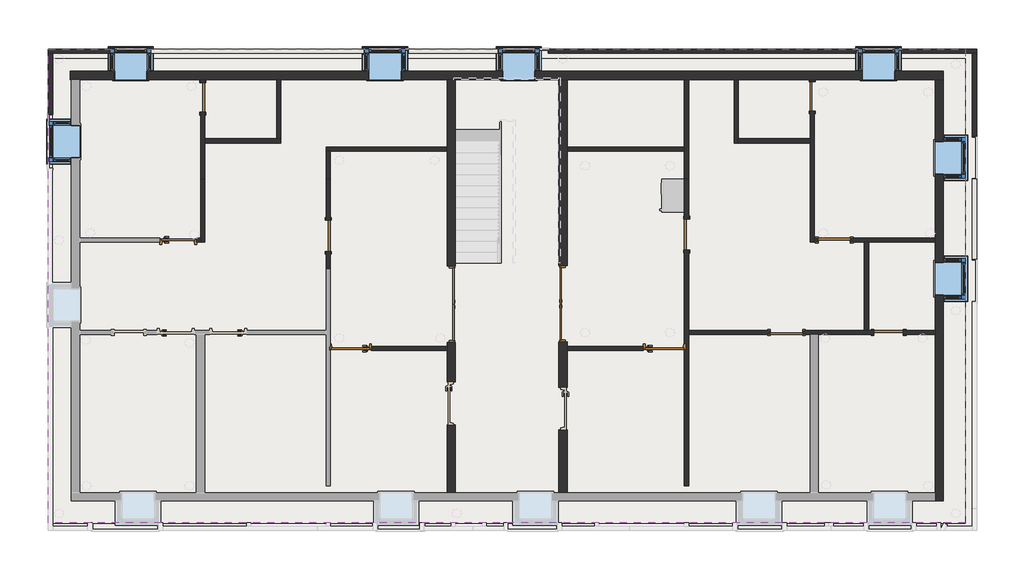
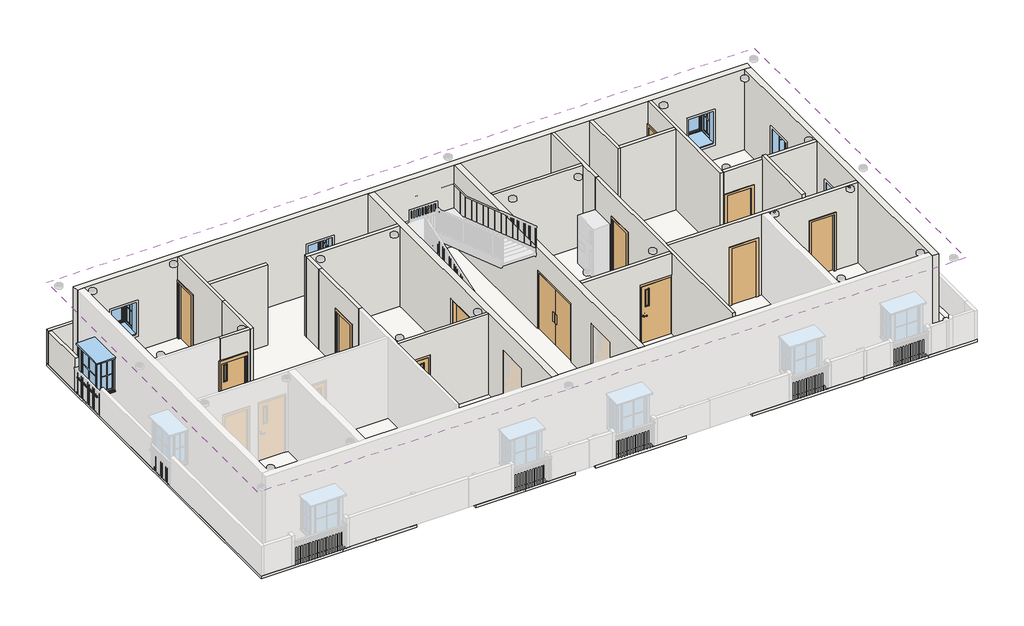
# One storey, part 2 of 7: 32 walls, 12 doors, 7 windows, 2 slabs, 1 covering.
"""IFC4 building model written with IfcOpenShell, lengths in millimetres."""

from ifc_helpers import new_model, si_unit, frame, origin, place, context, project, spatial, polyline, outline, extrude, faceted_brep, transform, mapped, element, save
from components import door_2c854dd0, door_cf1f2706, door_4f5842df, door_passage_single_vision_lite_3_x7_440dd290, door_70e57c00, door_700d3439, door_8cb1b8a7, door_38851409, door_d141acb4, window_bay_casement_box_90_degree_angle_center_fixed_4_x3_2dea7aab

model = new_model("IFC4")

# Units and contexts
model_context = context("Model", 3, world=origin())
ifc_project = project(units=[si_unit("LENGTHUNIT", "METRE", prefix="MILLI")], contexts=[model_context])

# Site, building, storey
site = spatial("IfcSite", under=ifc_project)
building = spatial("IfcBuilding", under=site)
storey = spatial("IfcBuildingStorey", under=building, Elevation=3200.4)

# Covering
placement = place(None, origin())
element("IfcCovering", 1, ObjectType="2' x 4' ACT System", at=placement, inside=storey, context=model_context, shape_type="SweptSolid", body=[
    extrude(outline(polyline([(12235.5012075, 8470.0067329), (12235.5012075, -4623.6932193), (-13088.8067989, -4623.6932193), (-13088.8067989, 8470.0067329), (12235.5012075, 8470.0067329)])), frame((0.0, 0.0, 6248.4), z_axis=(0.0, 0.0, 1.0), x_axis=(1.0, 0.0, 0.0)), (0.0, 0.0, 1.0), 57.15),
])

# Doors
door_shape = door_2c854dd0(model_context)
element("IfcDoor", 2, ObjectType="Door-Passage-Double-Flush-Dbl_Acting : 6'79\" X 84\"", at=placement, inside=storey, context=model_context, shape_type="MappedRepresentation", body=[
    mapped(door_shape, transform((-1969.4487998, 1424.4578621, 3200.4), x_axis=(0.0, -1.0, 0.0), y_axis=(1.0, 0.0, 0.0), z_axis=(0.0, 0.0, 1.0))),
])
element("IfcDoor", 3, ObjectType="Door-Passage-Double-Flush-Dbl_Acting : 6'79\" X 84\"", at=placement, inside=storey, context=model_context, shape_type="MappedRepresentation", body=[
    mapped(door_shape, transform((1128.8432011, 1434.2067807, 3200.4), x_axis=(0.0, 1.0, 0.0), y_axis=(-1.0, 0.0, 0.0), z_axis=(0.0, 0.0, 1.0))),
])
door_2_shape = door_cf1f2706(model_context)
element("IfcDoor", 4, ObjectType="Door-Passage-Single-Vision_Lite : 3'6\"X7' 2", at=placement, inside=storey, context=model_context, shape_type="MappedRepresentation", body=[
    mapped(door_2_shape, transform((-4750.7487995, 211.6078621, 3200.4), x_axis=(-1.0, 0.0, 0.0), y_axis=(0.0, -1.0, 0.0), z_axis=(0.0, 0.0, 1.0))),
])
door_3_shape = door_4f5842df(model_context)
element("IfcDoor", 5, ObjectType="Door-Passage-Single-Vision_Lite : 3'6\"X7' 2", at=placement, inside=storey, context=model_context, shape_type="MappedRepresentation", body=[
    mapped(door_3_shape, transform((3923.3512082, 211.6078621, 3200.4), x_axis=(1.0, 0.0, 0.0), y_axis=(0.0, 1.0, 0.0), z_axis=(0.0, 0.0, 1.0))),
])
door_passage_single_vision_lite_3_x7_shape = door_passage_single_vision_lite_3_x7_440dd290(model_context)
element("IfcDoor", 6, ObjectType="Door-Passage-Single-Vision_Lite : 3'X7'", at=placement, inside=storey, context=model_context, shape_type="MappedRepresentation", body=[
    mapped(door_passage_single_vision_lite_3_x7_shape, transform((-9501.8462614, 3186.8067332, 3200.4), x_axis=(1.0, 0.0, 0.0), y_axis=(0.0, 1.0, 0.0), z_axis=(0.0, 0.0, 1.0))),
])
door_4_shape = door_70e57c00(model_context)
element("IfcDoor", 7, ObjectType="Single-Flush : 2'10\" x 7'", at=placement, inside=storey, context=model_context, shape_type="MappedRepresentation", body=[
    mapped(door_4_shape, transform((-5360.3487995, 3313.8067802, 3200.4), x_axis=(0.0, -1.0, 0.0), y_axis=(1.0, 0.0, 0.0), z_axis=(0.0, 0.0, 1.0))),
])
door_5_shape = door_700d3439(model_context)
element("IfcDoor", 8, ObjectType="Single-Flush : 2'10\" x 7'", at=placement, inside=storey, context=model_context, shape_type="MappedRepresentation", body=[
    mapped(door_5_shape, transform((4532.9512082, 3351.906733, 3200.4), x_axis=(0.0, -1.0, 0.0), y_axis=(1.0, 0.0, 0.0), z_axis=(0.0, 0.0, 1.0))),
])
door_6_shape = door_8cb1b8a7(model_context)
element("IfcDoor", 9, ObjectType="Single-Flush : 2'11\"x 7'", at=placement, inside=storey, context=model_context, shape_type="MappedRepresentation", body=[
    mapped(door_6_shape, transform((8609.6512079, 3193.1567332, 3200.4), x_axis=(-1.0, 0.0, 0.0), y_axis=(0.0, -1.0, 0.0), z_axis=(0.0, 0.0, 1.0))),
])
element("IfcDoor", 10, ObjectType="Single-Flush : 2'11\"x 7'", at=placement, inside=storey, context=model_context, shape_type="MappedRepresentation", body=[
    mapped(door_6_shape, transform((7295.2012079, 640.4567334, 3200.4), x_axis=(1.0, 0.0, 0.0), y_axis=(0.0, 1.0, 0.0), z_axis=(0.0, 0.0, 1.0))),
])
door_7_shape = door_38851409(model_context)
element("IfcDoor", 11, ObjectType="Single-Flush : 2'8\"x 7'", at=placement, inside=storey, context=model_context, shape_type="MappedRepresentation", body=[
    mapped(door_7_shape, transform((-8827.4487992, 7136.5067329, 3200.4), x_axis=(0.0, 1.0, 0.0), y_axis=(-1.0, 0.0, 0.0), z_axis=(0.0, 0.0, 1.0))),
])
element("IfcDoor", 12, ObjectType="Single-Flush : 2'8\"x 7'", at=placement, inside=storey, context=model_context, shape_type="MappedRepresentation", body=[
    mapped(door_7_shape, transform((10111.5098918, 640.4567334, 3200.4), x_axis=(-1.0, 0.0, 0.0), y_axis=(0.0, -1.0, 0.0), z_axis=(0.0, 0.0, 1.0))),
])
door_8_shape = door_d141acb4(model_context)
element("IfcDoor", 13, ObjectType="Single-Flush : 2'8\"x 7'", at=placement, inside=storey, context=model_context, shape_type="MappedRepresentation", body=[
    mapped(door_8_shape, transform((8000.0512079, 7167.840939, 3200.4), x_axis=(0.0, 1.0, 0.0), y_axis=(-1.0, 0.0, 0.0), z_axis=(0.0, 0.0, 1.0))),
])

# Slabs
element("IfcSlab", 14, ObjectType="LW Concrete on Metal Deck", at=placement, inside=storey, context=model_context, shape_type="SweptSolid", body=[
    extrude(outline(polyline([(12235.5012075, 8203.3067329), (12235.5012075, -4623.6932193), (-12973.9987925, -4623.6932193), (-12973.9987925, 8203.3067329), (12235.5012075, 8203.3067329)])), frame((0.0, 0.0, 3095.625), z_axis=(0.0, 0.0, 1.0), x_axis=(1.0, 0.0, 0.0)), (0.0, 0.0, 1.0), 104.775),
])
element("IfcSlab", 15, ObjectType="LW Concrete on Metal Deck", at=placement, inside=storey, context=model_context, shape_type="SweptSolid", body=[
    extrude(outline(polyline([(12540.3012043, 8470.0067329), (12540.3012043, -4826.8932661), (10789.5617205, -4826.8932661), (8463.6012082, -4826.8932661), (8463.6012082, -3785.4932193), (8457.2512082, -3785.4932193), (8457.2512082, -4826.8932661), (4475.8012082, -4826.8932661), (4475.8012082, -3785.4932193), (2113.6012002, -3785.4932193), (2113.6012002, -4826.8932661), (-1112.1987998, -4826.8932661), (-1112.1987998, -3785.4932193), (-1848.7987998, -3785.4932193), (-1848.7987998, -4826.8932661), (-3627.0527957, -4826.8932661), (-5417.4987995, -4826.8932661), (-5417.4987995, -3785.4932193), (-7513.2527957, -3785.4932193), (-7513.2527957, -4826.8932661), (-8961.0527957, -4826.8932661), (-10167.8067989, -4826.8932661), (-13088.8067989, -4826.8932661), (-13088.8067989, 8470.0067329), (12540.3012043, 8470.0067329)])), frame((0.0, 0.0, 3095.625), z_axis=(0.0, 0.0, 1.0), x_axis=(1.0, 0.0, 0.0)), (0.0, 0.0, 1.0), 104.775),
])

# Walls
element("IfcWall", 16, ObjectType="Generic - 4.5\"", at=placement, inside=storey, context=model_context, shape_type="Brep", body=[
    faceted_brep([(-8884.5987992, 4875.906733, 3200.4), (-8884.5987992, 3250.3067332, 3200.4), (-8884.5987992, 3136.0067332, 3200.4), (-8884.5987992, 3136.0067332, 6248.4), (-8884.5987992, 3250.3067332, 6248.4), (-8884.5987992, 4875.906733, 6248.4), (-8770.2987992, 4875.906733, 3200.4), (-8770.2987992, 4875.906733, 6248.4), (-8770.2987992, 3136.0067332, 6248.4), (-8770.2987992, 3136.0067332, 3200.4)], [[[0, 1, 2, 3, 4, 5]], [[6, 7, 8, 9]], [[2, 1, 0, 6, 9]], [[5, 4, 3, 8, 7]], [[0, 5, 7, 6]], [[3, 2, 9, 8]]]),
])
element("IfcWall", 17, ObjectType="Generic - 4.5\"", at=placement, inside=storey, context=model_context, shape_type="SweptSolid", body=[
    extrude(outline(polyline([(6248.4, -2077.3987998), (6248.4, -5303.1987995), (5435.6, -5303.1987995), (5435.6, -4166.5487995), (3200.4, -4166.5487995), (3200.4, -2077.3987998), (6248.4, -2077.3987998)])), frame((0.0, 148.1078621, 0.0), z_axis=(0.0, 1.0, 0.0), x_axis=(0.0, 0.0, 1.0)), (0.0, 0.0, 1.0), 114.3),
])
element("IfcWall", 18, ObjectType="Generic - 4.5\"", at=placement, inside=storey, context=model_context, shape_type="Brep", body=[
    faceted_brep([(-2077.3987998, 5764.9067329, 3200.4), (-5417.4987995, 5764.9067329, 3200.4), (-5417.4987995, 5764.9067329, 6248.4), (-2077.3987998, 5764.9067329, 6248.4), (-2077.3987998, 5650.6067329, 3200.4), (-2077.3987998, 5650.6067329, 6248.4), (-5303.1987995, 5650.6067329, 6248.4), (-5417.4987995, 5650.6067329, 6248.4), (-5417.4987995, 5650.6067329, 3200.4), (-5303.1987995, 5650.6067329, 3200.4)], [[[0, 1, 2, 3]], [[4, 5, 6, 7, 8, 9]], [[1, 0, 4, 9, 8]], [[3, 2, 7, 6, 5]], [[2, 1, 8, 7]], [[0, 3, 5, 4]]]),
])
element("IfcWall", 19, ObjectType="Generic - 4.5\"", at=placement, inside=storey, context=model_context, shape_type="SweptSolid", body=[
    extrude(outline(polyline([(-5417.4987995, 4875.90678), (-5417.4987995, 5650.6067329), (-5303.1987995, 5650.6067329), (-5303.1987995, 4875.90678), (-5417.4987995, 4875.90678)])), frame((0.0, 0.0, 3200.4), z_axis=(0.0, 0.0, 1.0), x_axis=(1.0, 0.0, 0.0)), (0.0, 0.0, 1.0), 3048.0),
])
element("IfcWall", 20, ObjectType="Generic - 4.5\"", at=placement, inside=storey, context=model_context, shape_type="SweptSolid", body=[
    extrude(outline(polyline([(4475.8012082, 5650.6067329), (1250.0012085, 5650.6067329), (1250.0012085, 5764.9067329), (4475.8012082, 5764.9067329), (4475.8012082, 5650.6067329)])), frame((0.0, 0.0, 3200.4), z_axis=(0.0, 0.0, 1.0), x_axis=(1.0, 0.0, 0.0)), (0.0, 0.0, 1.0), 3048.0),
])
element("IfcWall", 21, ObjectType="Generic - 4.5\"", at=placement, inside=storey, context=model_context, shape_type="Brep", body=[
    faceted_brep([(4475.8012082, 7631.8067329, 3200.4), (4475.8012082, 5764.9067329, 3200.4), (4475.8012082, 5650.6067329, 3200.4), (4475.8012082, 4875.906733, 3200.4), (4475.8012082, 4875.906733, 6248.4), (4475.8012082, 5650.6067329, 6248.4), (4475.8012082, 5764.9067329, 6248.4), (4475.8012082, 7631.8067329, 6248.4), (4590.1012082, 7631.8067329, 3200.4), (4590.1012082, 7631.8067329, 6248.4), (4590.1012082, 4875.906733, 6248.4), (4590.1012082, 4875.906733, 3200.4)], [[[0, 1, 2, 3, 4, 5, 6, 7]], [[8, 9, 10, 11]], [[3, 2, 1, 0, 8, 11]], [[4, 3, 11, 10]], [[7, 6, 5, 4, 10, 9]], [[0, 7, 9, 8]]]),
])
element("IfcWall", 22, ObjectType="Generic - 4.5\"", at=placement, inside=storey, context=model_context, shape_type="Brep", body=[
    faceted_brep([(4475.8012082, -3594.9932193, 3200.4), (4475.8012082, -3594.9932193, 6248.4), (4475.8012082, 148.1078621, 6248.4), (4475.8012082, 262.4078621, 6248.4), (4475.8012082, 4875.906733, 6248.4), (4475.8012082, 4875.906733, 3200.4), (4475.8012082, 3783.706733, 3200.4), (4475.8012082, 3783.706733, 5334.0), (4475.8012082, 2920.106733, 5334.0), (4475.8012082, 2920.106733, 3200.4), (4475.8012082, 262.4078621, 3200.4), (4475.8012082, 262.4078621, 5435.6), (4475.8012082, 148.1078621, 5435.6), (4475.8012082, 148.1078621, 3200.4), (4590.1012082, -3594.9932193, 6248.4), (4590.1012082, -3594.9932193, 3200.4), (4590.1012082, 583.3067334, 3200.4), (4590.1012082, 697.6067334, 3200.4), (4590.1012082, 2920.106733, 3200.4), (4590.1012082, 2920.106733, 5334.0), (4590.1012082, 3783.706733, 5334.0), (4590.1012082, 3783.706733, 3200.4), (4590.1012082, 4875.906733, 3200.4), (4590.1012082, 4875.906733, 6248.4), (4590.1012082, 697.6067334, 6248.4), (4590.1012082, 583.3067334, 6248.4), (4507.5512082, 148.1078621, 3200.4), (4507.5512082, 262.4078621, 3200.4), (4507.5512082, 148.1078621, 5435.6), (4507.5512082, 262.4078621, 5435.6)], [[[0, 1, 2, 3, 4, 5, 6, 7, 8, 9, 10, 11, 12, 13]], [[14, 15, 16, 17, 18, 19, 20, 21, 22, 23, 24, 25]], [[15, 0, 13, 26, 27, 10, 9, 18, 17, 16]], [[5, 22, 21, 6]], [[1, 0, 15, 14]], [[4, 3, 2, 1, 14, 25, 24, 23]], [[5, 4, 23, 22]], [[19, 18, 9, 8]], [[20, 19, 8, 7]], [[21, 20, 7, 6]], [[28, 26, 13, 12]], [[27, 29, 11, 10]], [[26, 28, 29, 27]], [[29, 28, 12, 11]]]),
])
element("IfcWall", 23, ObjectType="Generic - 4.5\"", at=placement, inside=storey, context=model_context, shape_type="Brep", body=[
    faceted_brep([(5847.401208, 7631.8067329, 3200.4), (5847.401208, 5879.2067329, 3200.4), (5847.401208, 5879.2067329, 6248.4), (5847.401208, 7631.8067329, 6248.4), (5961.701208, 7631.8067329, 3200.4), (5961.701208, 7631.8067329, 6248.4), (5961.701208, 5993.5067329, 6248.4), (5961.701208, 5879.2067329, 6248.4), (5961.701208, 5879.2067329, 3200.4), (5961.701208, 5993.5067329, 3200.4)], [[[0, 1, 2, 3]], [[4, 5, 6, 7, 8, 9]], [[1, 0, 4, 9, 8]], [[3, 2, 7, 6, 5]], [[0, 3, 5, 4]], [[2, 1, 8, 7]]]),
])
element("IfcWall", 24, ObjectType="Generic - 4.5\"", at=placement, inside=storey, context=model_context, shape_type="SweptSolid", body=[
    extrude(outline(polyline([(7942.9012079, 5879.2067329), (5961.701208, 5879.2067329), (5961.701208, 5993.5067329), (7942.9012079, 5993.5067329), (7942.9012079, 5879.2067329)])), frame((0.0, 0.0, 3200.4), z_axis=(0.0, 0.0, 1.0), x_axis=(1.0, 0.0, 0.0)), (0.0, 0.0, 1.0), 3048.0),
])
element("IfcWall", 25, ObjectType="Generic - 4.5\"", at=placement, inside=storey, context=model_context, shape_type="Brep", body=[
    faceted_brep([(7942.9012079, 7625.040939, 3200.4), (7942.9012079, 7574.240939, 3200.4), (7942.9012079, 7574.240939, 5334.0), (7942.9012079, 6761.440939, 5334.0), (7942.9012079, 6761.440939, 3200.4), (7942.9012079, 5993.5067329, 3200.4), (7942.9012079, 5879.2067329, 3200.4), (7942.9012079, 3136.0067332, 3200.4), (7942.9012079, 3136.0067332, 6248.4), (7942.9012079, 5879.2067329, 6248.4), (7942.9012079, 5993.5067329, 6248.4), (7942.9012079, 7625.040939, 6248.4), (8057.2012079, 7574.240939, 5334.0), (8057.2012079, 7574.240939, 3200.4), (8057.2012079, 7625.040939, 3200.4), (8057.2012079, 7625.040939, 6248.4), (8057.2012079, 3250.3067332, 6248.4), (8057.2012079, 3136.0067332, 6248.4), (8057.2012079, 3136.0067332, 3200.4), (8057.2012079, 3250.3067332, 3200.4), (8057.2012079, 6761.440939, 3200.4), (8057.2012079, 6761.440939, 5334.0)], [[[0, 1, 2, 3, 4, 5, 6, 7, 8, 9, 10, 11]], [[12, 13, 14, 15, 16, 17, 18, 19, 20, 21]], [[14, 13, 1, 0]], [[20, 19, 18, 7, 6, 5, 4]], [[11, 10, 9, 8, 17, 16, 15]], [[0, 11, 15, 14]], [[8, 7, 18, 17]], [[2, 1, 13, 12]], [[3, 2, 12, 21]], [[4, 3, 21, 20]]]),
])
element("IfcWall", 26, ObjectType="Generic - 4.5\"", at=placement, inside=storey, context=model_context, shape_type="Brep", body=[
    faceted_brep([(8165.1512079, 3250.3067332, 5334.0), (8165.1512079, 3250.3067332, 3200.4), (8057.2012079, 3250.3067332, 3200.4), (8057.2012079, 3250.3067332, 6248.4), (11397.3012075, 3250.3067332, 6248.4), (11397.3012075, 3250.3067332, 3200.4), (9054.1512079, 3250.3067332, 3200.4), (9054.1512079, 3250.3067332, 5334.0), (8057.2012079, 3136.0067332, 3200.4), (8165.1512079, 3136.0067332, 3200.4), (8165.1512079, 3136.0067332, 5334.0), (9054.1512079, 3136.0067332, 5334.0), (9054.1512079, 3136.0067332, 3200.4), (9438.4098918, 3136.0067332, 3200.4), (9565.4098918, 3136.0067332, 3200.4), (11397.3012075, 3136.0067332, 3200.4), (11397.3012075, 3136.0067332, 6248.4), (8057.2012079, 3136.0067332, 6248.4)], [[[0, 1, 2, 3, 4, 5, 6, 7]], [[8, 9, 10, 11, 12, 13, 14, 15, 16, 17]], [[6, 5, 15, 14, 13, 12]], [[2, 1, 9, 8]], [[4, 3, 17, 16]], [[3, 2, 8, 17]], [[5, 4, 16, 15]], [[10, 9, 1, 0]], [[11, 10, 0, 7]], [[12, 11, 7, 6]]]),
])
element("IfcWall", 27, ObjectType="Generic - 4.5\"", at=placement, inside=storey, context=model_context, shape_type="Brep", body=[
    faceted_brep([(7739.7012079, 583.3067334, 5334.0), (7739.7012079, 583.3067334, 3200.4), (7942.9012079, 583.3067334, 3200.4), (8171.5012079, 583.3067334, 3200.4), (9705.1098918, 583.3067334, 3200.4), (9705.1098918, 583.3067334, 5334.0), (10517.9098918, 583.3067334, 5334.0), (10517.9098918, 583.3067334, 3200.4), (11397.3012075, 583.3067334, 3200.4), (11397.3012075, 583.3067334, 6248.4), (8171.5012079, 583.3067334, 6248.4), (7942.9012079, 583.3067334, 6248.4), (4590.1012082, 583.3067334, 6248.4), (4590.1012082, 583.3067334, 3200.4), (6850.7012079, 583.3067334, 3200.4), (6850.7012079, 583.3067334, 5334.0), (9705.1098918, 697.6067334, 3200.4), (9565.4098918, 697.6067334, 3200.4), (9438.4098918, 697.6067334, 3200.4), (7739.7012079, 697.6067334, 3200.4), (7739.7012079, 697.6067334, 5334.0), (6850.7012079, 697.6067334, 5334.0), (6850.7012079, 697.6067334, 3200.4), (4590.1012082, 697.6067334, 3200.4), (4590.1012082, 697.6067334, 6248.4), (11397.3012075, 697.6067334, 6248.4), (11397.3012075, 697.6067334, 3200.4), (10517.9098918, 697.6067334, 3200.4), (10517.9098918, 697.6067334, 5334.0), (9705.1098918, 697.6067334, 5334.0)], [[[0, 1, 2, 3, 4, 5, 6, 7, 8, 9, 10, 11, 12, 13, 14, 15]], [[16, 17, 18, 19, 20, 21, 22, 23, 24, 25, 26, 27, 28, 29]], [[27, 26, 8, 7]], [[14, 13, 23, 22]], [[4, 3, 2, 1, 19, 18, 17, 16]], [[12, 11, 10, 9, 25, 24]], [[9, 8, 26, 25]], [[13, 12, 24, 23]], [[5, 4, 16, 29]], [[6, 5, 29, 28]], [[7, 6, 28, 27]], [[20, 19, 1, 0]], [[21, 20, 0, 15]], [[22, 21, 15, 14]]]),
])
element("IfcWall", 28, ObjectType="Generic - 4.5\"", at=placement, inside=storey, context=model_context, shape_type="Brep", body=[
    faceted_brep([(-8770.2987992, 7542.9067329, 5334.0), (-8770.2987992, 7542.9067329, 3200.4), (-8770.2987992, 7631.8067329, 3200.4), (-8770.2987992, 7631.8067329, 6248.4), (-8770.2987992, 5993.5067329, 6248.4), (-8770.2987992, 5879.2067329, 6248.4), (-8770.2987992, 4875.906733, 6248.4), (-8770.2987992, 4875.906733, 3200.4), (-8770.2987992, 5879.2067329, 3200.4), (-8770.2987992, 5993.5067329, 3200.4), (-8770.2987992, 6730.1067329, 3200.4), (-8770.2987992, 6730.1067329, 5334.0), (-8884.5987992, 7631.8067329, 3200.4), (-8884.5987992, 7542.9067329, 3200.4), (-8884.5987992, 7542.9067329, 5334.0), (-8884.5987992, 6730.1067329, 5334.0), (-8884.5987992, 6730.1067329, 3200.4), (-8884.5987992, 4875.906733, 3200.4), (-8884.5987992, 4875.906733, 6248.4), (-8884.5987992, 7631.8067329, 6248.4)], [[[0, 1, 2, 3, 4, 5, 6, 7, 8, 9, 10, 11]], [[12, 13, 14, 15, 16, 17, 18, 19]], [[2, 1, 13, 12]], [[10, 9, 8, 7, 17, 16]], [[6, 5, 4, 3, 19, 18]], [[7, 6, 18, 17]], [[3, 2, 12, 19]], [[14, 13, 1, 0]], [[15, 14, 0, 11]], [[16, 15, 11, 10]]]),
])
element("IfcWall", 29, ObjectType="Generic - 4.5\"", at=placement, inside=storey, context=model_context, shape_type="Brep", body=[
    faceted_brep([(-8770.2987992, 5879.2067329, 3200.4), (-6674.7987994, 5879.2067329, 3200.4), (-6674.7987994, 5879.2067329, 6248.4), (-8770.2987992, 5879.2067329, 6248.4), (-8770.2987992, 5993.5067329, 3200.4), (-8770.2987992, 5993.5067329, 6248.4), (-6674.7987994, 5993.5067329, 6248.4), (-6674.7987994, 5993.5067329, 4572.0), (-6674.7987994, 5993.5067329, 3200.4), (-6789.0987994, 5993.5067329, 3200.4)], [[[0, 1, 2, 3]], [[4, 5, 6, 7, 8, 9]], [[1, 0, 4, 9, 8]], [[3, 2, 6, 5]], [[0, 3, 5, 4]], [[2, 1, 8, 7, 6]]]),
])
element("IfcWall", 30, ObjectType="Generic - 4.5\"", at=placement, inside=storey, context=model_context, shape_type="SweptSolid", body=[
    extrude(outline(polyline([(-6674.7987994, 7631.8067329), (-6674.7987994, 5993.5067329), (-6789.0987994, 5993.5067329), (-6789.0987994, 7631.8067329), (-6674.7987994, 7631.8067329)])), frame((0.0, 0.0, 3200.4), z_axis=(0.0, 0.0, 1.0), x_axis=(1.0, 0.0, 0.0)), (0.0, 0.0, 1.0), 1371.6),
])
element("IfcWall", 31, ObjectType="Generic - 4.5\"", at=placement, inside=storey, context=model_context, shape_type="SweptSolid", body=[
    extrude(outline(polyline([(6248.4, -8884.5987992), (6248.4, -9959.0462614), (5435.6, -9959.0462614), (5435.6, -8993.8462614), (3200.4, -8993.8462614), (3200.4, -8884.5987992), (6248.4, -8884.5987992)])), frame((0.0, 3136.0067332, 0.0), z_axis=(0.0, 1.0, 0.0), x_axis=(0.0, 0.0, 1.0)), (0.0, 0.0, 1.0), 114.3),
])
element("IfcWall", 32, ObjectType="Generic - 4.5\"", at=placement, inside=storey, context=model_context, shape_type="SweptSolid", body=[
    extrude(outline(polyline([(2882.0067802, 5334.0), (2882.0067802, 3200.4), (2399.4067802, 3200.4), (2399.4067802, 6248.4), (4875.90678, 6248.4), (4875.90678, 3200.4), (3745.6067802, 3200.4), (3745.6067802, 5334.0), (2882.0067802, 5334.0)])), frame((-5417.4987995, 0.0, 0.0), z_axis=(1.0, 0.0, 0.0), x_axis=(0.0, 1.0, 0.0)), (0.0, 0.0, 1.0), 114.3),
])
element("IfcWall", 33, ObjectType="Generic - 4.5\"", at=placement, inside=storey, context=model_context, shape_type="SweptSolid", body=[
    extrude(outline(polyline([(6248.4, 4475.8012082), (6248.4, 1250.0012085), (3200.4, 1250.0012085), (3200.4, 3339.1512082), (5435.6, 3339.1512082), (5435.6, 4475.8012082), (6248.4, 4475.8012082)])), frame((0.0, 148.1078621, 0.0), z_axis=(0.0, 1.0, 0.0), x_axis=(0.0, 0.0, 1.0)), (0.0, 0.0, 1.0), 114.3),
])
element("IfcWall", 34, ObjectType="Generic - 4.5\"", at=placement, inside=storey, context=model_context, shape_type="SweptSolid", body=[
    extrude(outline(polyline([(-12973.9987925, 8355.7067329), (-12973.9987925, 6682.2711337), (-13088.2987925, 6682.2711337), (-13088.2987925, 8355.7067329), (-12973.9987925, 8355.7067329)])), frame((0.0, 0.0, 3200.4), z_axis=(0.0, 0.0, 1.0), x_axis=(1.0, 0.0, 0.0)), (0.0, 0.0, 1.0), 1259.0059812),
])
element("IfcWall", 35, ObjectType="Generic - 4.5\"", at=placement, inside=storey, context=model_context, shape_type="Brep", body=[
    faceted_brep([(-13088.8067989, 8355.7067329, 3200.4), (-13088.2987925, 8355.7067329, 3200.4), (-12973.9987925, 8355.7067329, 3200.4), (-11387.0067989, 8355.7067329, 3200.4), (-11387.0067989, 8355.7067329, 4473.8134002), (-13088.8067989, 8355.7067329, 4473.8134002), (-13088.8067989, 8470.0067329, 3200.4), (-13088.8067989, 8470.0067329, 4473.8134002), (-11387.0067989, 8470.0067329, 4473.8134002), (-11387.0067989, 8470.0067329, 3200.4)], [[[0, 1, 2, 3, 4, 5]], [[6, 7, 8, 9]], [[3, 2, 1, 0, 6, 9]], [[4, 3, 9, 8]], [[5, 4, 8, 7]], [[0, 5, 7, 6]]]),
])
element("IfcWall", 36, ObjectType="Generic - 4.5\"", at=placement, inside=storey, context=model_context, shape_type="SweptSolid", body=[
    extrude(outline(polyline([(-4382.4487992, 8355.7067329), (-10247.1817989, 8355.7067329), (-10247.1817989, 8470.0067329), (-4382.4487992, 8470.0067329), (-4382.4487992, 8355.7067329)])), frame((0.0, 0.0, 3200.4), z_axis=(0.0, 0.0, 1.0), x_axis=(1.0, 0.0, 0.0)), (0.0, 0.0, 1.0), 1083.89837),
])
element("IfcWall", 37, ObjectType="Generic - 4.5\"", at=placement, inside=storey, context=model_context, shape_type="SweptSolid", body=[
    extrude(outline(polyline([(-682.0490672, 8355.7067329), (-3139.4990672, 8355.7067329), (-3139.4990672, 8470.0067329), (-682.0490672, 8470.0067329), (-682.0490672, 8355.7067329)])), frame((0.0, 0.0, 3200.4), z_axis=(0.0, 0.0, 1.0), x_axis=(1.0, 0.0, 0.0)), (0.0, 0.0, 1.0), 1195.9732529),
])
element("IfcWall", 38, ObjectType="Generic - 4.5\"", at=placement, inside=storey, context=model_context, shape_type="SweptSolid", body=[
    extrude(outline(polyline([(9199.6932011, 8355.7067329), (741.4932011, 8355.7067329), (741.4932011, 8470.0067329), (9199.6932011, 8470.0067329), (9199.6932011, 8355.7067329)])), frame((0.0, 0.0, 3200.4), z_axis=(0.0, 0.0, 1.0), x_axis=(1.0, 0.0, 0.0)), (0.0, 0.0, 1.0), 1274.1868366),
])
element("IfcWall", 39, ObjectType="Generic - 4.5\"", at=placement, inside=storey, context=model_context, shape_type="Brep", body=[
    faceted_brep([(10462.2009401, 8355.7067329, 3200.4), (12426.0012043, 8355.7067329, 3200.4), (12540.3012043, 8355.7067329, 3200.4), (12540.3012043, 8355.7067329, 4566.1502881), (10462.2009401, 8355.7067329, 4566.1502881), (10462.2009401, 8470.0067329, 3200.4), (10462.2009401, 8470.0067329, 4566.1502881), (12540.3012043, 8470.0067329, 4566.1502881), (12540.3012043, 8470.0067329, 3200.4)], [[[0, 1, 2, 3, 4]], [[5, 6, 7, 8]], [[2, 1, 0, 5, 8]], [[4, 3, 7, 6]], [[0, 4, 6, 5]], [[3, 2, 8, 7]]]),
])
element("IfcWall", 40, ObjectType="Generic - 4.5\"", at=placement, inside=storey, context=model_context, shape_type="Brep", body=[
    faceted_brep([(12426.0012043, 8355.7067329, 3200.4), (12426.0012043, 6069.7067329, 3200.4), (12426.0012043, 6069.7067329, 4572.0), (12426.0012043, 8355.7067329, 4572.0), (12540.3012043, 8355.7067329, 3200.4), (12540.3012043, 8355.7067329, 4566.1502881), (12540.3012043, 8355.7067329, 4572.0), (12540.3012043, 6069.7067329, 4572.0), (12540.3012043, 6069.7067329, 3200.4)], [[[0, 1, 2, 3]], [[4, 5, 6, 7, 8]], [[1, 0, 4, 8]], [[2, 1, 8, 7]], [[3, 2, 7, 6]], [[0, 3, 6, 5, 4]]]),
])
element("IfcWall", 41, ObjectType="Generic - 4.5\"", at=placement, inside=storey, context=model_context, shape_type="SweptSolid", body=[
    extrude(outline(polyline([(12426.0012043, 2666.1067329), (12426.0012043, 4875.9067329), (12540.3012043, 4875.9067329), (12540.3012043, 2666.1067329), (12426.0012043, 2666.1067329)])), frame((0.0, 0.0, 3200.4), z_axis=(0.0, 0.0, 1.0), x_axis=(1.0, 0.0, 0.0)), (0.0, 0.0, 1.0), 1193.0409005),
])
element("IfcWall", 42, ObjectType="Generic - 9\"", at=placement, inside=storey, context=model_context, shape_type="Brep", body=[
    faceted_brep([(-12479.2067989, 7631.8067329, 3200.4), (-12453.2987925, 7631.8067329, 3200.4), (-12224.6987925, 7631.8067329, 3200.4), (-8884.5987992, 7631.8067329, 3200.4), (-8770.2987992, 7631.8067329, 3200.4), (-6789.0987994, 7631.8067329, 3200.4), (-6674.7987994, 7631.8067329, 3200.4), (-2077.3987998, 7631.8067329, 3200.4), (-1848.7987998, 7631.8067329, 3200.4), (1008.1932011, 7631.8067329, 3200.4), (1236.7932011, 7631.8067329, 3200.4), (4475.8012082, 7631.8067329, 3200.4), (4590.1012082, 7631.8067329, 3200.4), (5847.401208, 7631.8067329, 3200.4), (5961.701208, 7631.8067329, 3200.4), (11397.3012075, 7631.8067329, 3200.4), (11625.9012075, 7631.8067329, 3200.4), (11625.9012075, 7631.8067329, 6248.4), (11397.3012075, 7631.8067329, 6248.4), (5961.701208, 7631.8067329, 6248.4), (5847.401208, 7631.8067329, 6248.4), (4590.1012082, 7631.8067329, 6248.4), (4475.8012082, 7631.8067329, 6248.4), (1236.7932011, 7631.8067329, 6248.4), (1008.1932011, 7631.8067329, 6248.4), (-1848.7987998, 7631.8067329, 6248.4), (-2077.3987998, 7631.8067329, 6248.4), (-8770.2987992, 7631.8067329, 6248.4), (-8884.5987992, 7631.8067329, 6248.4), (-12224.6987925, 7631.8067329, 6248.4), (-12453.2987925, 7631.8067329, 6248.4), (-12479.2067989, 7631.8067329, 6248.4), (-10357.7987925, 7631.8067329, 5080.0), (-10357.7987925, 7631.8067329, 3810.0), (-11272.1987925, 7631.8067329, 3810.0), (-11272.1987925, 7631.8067329, 5080.0), (-3334.6987998, 7631.8067329, 5080.0), (-3334.6987998, 7631.8067329, 3810.0), (-4249.0987998, 7631.8067329, 3810.0), (-4249.0987998, 7631.8067329, 5080.0), (360.4932011, 7631.8067329, 5080.0), (360.4932011, 7631.8067329, 3810.0), (-553.9067989, 7631.8067329, 3810.0), (-553.9067989, 7631.8067329, 5080.0), (10292.4012075, 7631.8067329, 5080.0), (10292.4012075, 7631.8067329, 3810.0), (9378.0012075, 7631.8067329, 3810.0), (9378.0012075, 7631.8067329, 5080.0), (-12479.2067989, 7860.4067329, 3200.4), (-12479.2067989, 7860.4067329, 6248.4), (11625.9012075, 7860.4067329, 6248.4), (11625.9012075, 7860.4067329, 3200.4), (-10357.7987925, 7860.4067329, 5080.0), (-11272.1987925, 7860.4067329, 5080.0), (-11272.1987925, 7860.4067329, 3810.0), (-10357.7987925, 7860.4067329, 3810.0), (-3334.6987998, 7860.4067329, 5080.0), (-4249.0987998, 7860.4067329, 5080.0), (-4249.0987998, 7860.4067329, 3810.0), (-3334.6987998, 7860.4067329, 3810.0), (360.4932011, 7860.4067329, 5080.0), (-553.9067989, 7860.4067329, 5080.0), (-553.9067989, 7860.4067329, 3810.0), (360.4932011, 7860.4067329, 3810.0), (10292.4012075, 7860.4067329, 5080.0), (9378.0012075, 7860.4067329, 5080.0), (9378.0012075, 7860.4067329, 3810.0), (10292.4012075, 7860.4067329, 3810.0)], [[[0, 1, 2, 3, 4, 5, 6, 7, 8, 9, 10, 11, 12, 13, 14, 15, 16, 17, 18, 19, 20, 21, 22, 23, 24, 25, 26, 27, 28, 29, 30, 31], [32, 33, 34, 35], [36, 37, 38, 39], [40, 41, 42, 43], [44, 45, 46, 47]], [[48, 49, 50, 51], [52, 53, 54, 55], [56, 57, 58, 59], [60, 61, 62, 63], [64, 65, 66, 67]], [[16, 15, 14, 13, 12, 11, 10, 9, 8, 7, 6, 5, 4, 3, 2, 1, 0, 48, 51]], [[31, 30, 29, 28, 27, 26, 25, 24, 23, 22, 21, 20, 19, 18, 17, 50, 49]], [[0, 31, 49, 48]], [[17, 16, 51, 50]], [[33, 32, 52, 55]], [[34, 33, 55, 54]], [[35, 34, 54, 53]], [[32, 35, 53, 52]], [[37, 36, 56, 59]], [[38, 37, 59, 58]], [[39, 38, 58, 57]], [[36, 39, 57, 56]], [[41, 40, 60, 63]], [[42, 41, 63, 62]], [[43, 42, 62, 61]], [[40, 43, 61, 60]], [[45, 44, 64, 67]], [[46, 45, 67, 66]], [[47, 46, 66, 65]], [[44, 47, 65, 64]]]),
])
element("IfcWall", 43, ObjectType="Generic - 9\"", at=placement, inside=storey, context=model_context, shape_type="Brep", body=[
    faceted_brep([(11397.3012075, 7631.8067329, 3200.4), (11397.3012075, 3250.3067332, 3200.4), (11397.3012075, 3136.0067332, 3200.4), (11397.3012075, 697.6067334, 3200.4), (11397.3012075, 583.3067334, 3200.4), (11397.3012075, -3785.4932193, 3200.4), (11397.3012075, -4014.0932193, 3200.4), (11397.3012075, -4014.0932193, 6248.4), (11397.3012075, -3785.4932193, 6248.4), (11397.3012075, 583.3067334, 6248.4), (11397.3012075, 697.6067334, 6248.4), (11397.3012075, 3136.0067332, 6248.4), (11397.3012075, 3250.3067332, 6248.4), (11397.3012075, 7631.8067329, 6248.4), (11397.3012075, 1669.1567332, 5080.0), (11397.3012075, 1669.1567332, 3810.0), (11397.3012075, 2583.5567332, 3810.0), (11397.3012075, 2583.5567332, 5080.0), (11397.3012075, 5012.431733, 5080.0), (11397.3012075, 5012.431733, 3810.0), (11397.3012075, 5926.831733, 3810.0), (11397.3012075, 5926.831733, 5080.0), (11625.9012075, 7631.8067329, 3200.4), (11625.9012075, 7631.8067329, 6248.4), (11625.9012075, -4014.0932193, 6248.4), (11625.9012075, -4014.0932193, 3200.4), (11625.9012075, 1669.1567332, 5080.0), (11625.9012075, 2583.5567332, 5080.0), (11625.9012075, 2583.5567332, 3810.0), (11625.9012075, 1669.1567332, 3810.0), (11625.9012075, 5012.431733, 5080.0), (11625.9012075, 5926.831733, 5080.0), (11625.9012075, 5926.831733, 3810.0), (11625.9012075, 5012.431733, 3810.0)], [[[0, 1, 2, 3, 4, 5, 6, 7, 8, 9, 10, 11, 12, 13], [14, 15, 16, 17], [18, 19, 20, 21]], [[22, 23, 24, 25], [26, 27, 28, 29], [30, 31, 32, 33]], [[6, 5, 4, 3, 2, 1, 0, 22, 25]], [[13, 12, 11, 10, 9, 8, 7, 24, 23]], [[0, 13, 23, 22]], [[7, 6, 25, 24]], [[15, 14, 26, 29]], [[16, 15, 29, 28]], [[17, 16, 28, 27]], [[14, 17, 27, 26]], [[19, 18, 30, 33]], [[20, 19, 33, 32]], [[21, 20, 32, 31]], [[18, 21, 31, 30]]]),
])
element("IfcWall", 44, ObjectType="Generic - 9\"", at=placement, inside=storey, context=model_context, shape_type="Brep", body=[
    faceted_brep([(-2077.3987998, -3785.4932193, 6248.4), (-2077.3987998, 148.1078621, 6248.4), (-2077.3987998, 262.4078621, 6248.4), (-2077.3987998, 5650.6067329, 6248.4), (-2077.3987998, 5764.9067329, 6248.4), (-2077.3987998, 7631.8067329, 6248.4), (-2077.3987998, 7631.8067329, 3200.4), (-2077.3987998, 5764.9067329, 3200.4), (-2077.3987998, 5650.6067329, 3200.4), (-2077.3987998, 2478.5578621, 3200.4), (-2077.3987998, 2478.5578621, 5435.6), (-2077.3987998, 370.3578621, 5435.6), (-2077.3987998, 370.3578621, 3200.4), (-2077.3987998, 262.4078621, 3200.4), (-2077.3987998, 148.1078621, 3200.4), (-2077.3987998, -721.8421379, 3200.4), (-2077.3987998, -721.8421379, 5435.6), (-2077.3987998, -1915.6421379, 5435.6), (-2077.3987998, -1915.6421379, 3200.4), (-2077.3987998, -3785.4932193, 3200.4), (-1848.7987998, 7631.8067329, 6248.4), (-1848.7987998, -3785.4932193, 6248.4), (-1848.7987998, -3785.4932193, 3200.4), (-1848.7987998, -1915.6421379, 3200.4), (-1848.7987998, -1915.6421379, 5435.6), (-1848.7987998, -721.8421379, 5435.6), (-1848.7987998, -721.8421379, 3200.4), (-1848.7987998, 370.3578621, 3200.4), (-1848.7987998, 370.3578621, 5435.6), (-1848.7987998, 2478.5578621, 5435.6), (-1848.7987998, 2478.5578621, 3200.4), (-1848.7987998, 7631.8067329, 3200.4)], [[[0, 1, 2, 3, 4, 5, 6, 7, 8, 9, 10, 11, 12, 13, 14, 15, 16, 17, 18, 19]], [[20, 21, 22, 23, 24, 25, 26, 27, 28, 29, 30, 31]], [[22, 19, 18, 23]], [[6, 31, 30, 9, 8, 7]], [[26, 15, 14, 13, 12, 27]], [[5, 4, 3, 2, 1, 0, 21, 20]], [[0, 19, 22, 21]], [[6, 5, 20, 31]], [[17, 24, 23, 18]], [[24, 17, 16, 25]], [[25, 16, 15, 26]], [[11, 28, 27, 12]], [[28, 11, 10, 29]], [[29, 10, 9, 30]]]),
])
element("IfcWall", 45, ObjectType="Generic - 9\"", at=placement, inside=storey, context=model_context, shape_type="SweptSolid", body=[
    extrude(outline(polyline([(-3785.4932193, 6248.4), (7631.8067329, 6248.4), (7631.8067329, 3200.4), (2488.3067807, 3200.4), (2488.3067807, 5435.6), (380.1067807, 5435.6), (380.1067807, 3200.4), (-877.1932193, 3200.4), (-877.1932193, 5435.6), (-2045.5932193, 5435.6), (-2045.5932193, 3200.4), (-3785.4932193, 3200.4), (-3785.4932193, 6248.4)])), frame((1008.1932011, 0.0, 0.0), z_axis=(1.0, 0.0, 0.0), x_axis=(0.0, 1.0, 0.0)), (0.0, 0.0, 1.0), 228.6),
])
element("IfcWall", 46, ObjectType="Interior - 5\" Partition (2-hr)", at=placement, inside=storey, context=model_context, shape_type="SweptSolid", body=[
    extrude(outline(polyline([(9438.4098918, 697.6067334), (9438.4098918, 3136.0067332), (9565.4098918, 3136.0067332), (9565.4098918, 697.6067334), (9438.4098918, 697.6067334)])), frame((0.0, 0.0, 3200.4), z_axis=(0.0, 0.0, 1.0), x_axis=(1.0, 0.0, 0.0)), (0.0, 0.0, 1.0), 3200.4),
])
element("IfcWall", 47, ObjectType="Interior - 5\" Partition (2-hr)", at=placement, inside=storey, context=model_context, shape_type="SweptSolid", body=[
    extrude(outline(polyline([(9438.4098918, 697.6067334), (9438.4098918, 3136.0067332), (9565.4098918, 3136.0067332), (9565.4098918, 697.6067334), (9438.4098918, 697.6067334)])), frame((0.0, 0.0, 3200.4), z_axis=(0.0, 0.0, 1.0), x_axis=(1.0, 0.0, 0.0)), (0.0, 0.0, 1.0), 3200.4),
])

# Windows
window_bay_casement_box_90_degree_angle_center_fixed_4_x3_shape = window_bay_casement_box_90_degree_angle_center_fixed_4_x3_2dea7aab(model_context)
element("IfcWindow", 48, ObjectType="Window-Bay-Casement-Box-90_Degree_Angle-Center_Fixed : 4'X3'", at=placement, inside=storey, context=model_context, shape_type="MappedRepresentation", body=[
    mapped(window_bay_casement_box_90_degree_angle_center_fixed_4_x3_shape, transform((-10814.9987925, 7746.1067329, 3200.4), x_axis=(1.0, 0.0, 0.0), y_axis=(0.0, 1.0, 0.0), z_axis=(0.0, 0.0, 1.0))),
])
element("IfcWindow", 49, ObjectType="Window-Bay-Casement-Box-90_Degree_Angle-Center_Fixed : 4'X3'", at=placement, inside=storey, context=model_context, shape_type="MappedRepresentation", body=[
    mapped(window_bay_casement_box_90_degree_angle_center_fixed_4_x3_shape, transform((-3791.8987998, 7746.1067329, 3200.4), x_axis=(1.0, 0.0, 0.0), y_axis=(0.0, 1.0, 0.0), z_axis=(0.0, 0.0, 1.0))),
])
element("IfcWindow", 50, ObjectType="Window-Bay-Casement-Box-90_Degree_Angle-Center_Fixed : 4'X3'", at=placement, inside=storey, context=model_context, shape_type="MappedRepresentation", body=[
    mapped(window_bay_casement_box_90_degree_angle_center_fixed_4_x3_shape, transform((-96.7067989, 7746.1067329, 3200.4), x_axis=(1.0, 0.0, 0.0), y_axis=(0.0, 1.0, 0.0), z_axis=(0.0, 0.0, 1.0))),
])
element("IfcWindow", 51, ObjectType="Window-Bay-Casement-Box-90_Degree_Angle-Center_Fixed : 4'X3'", at=placement, inside=storey, context=model_context, shape_type="MappedRepresentation", body=[
    mapped(window_bay_casement_box_90_degree_angle_center_fixed_4_x3_shape, transform((9835.2012075, 7746.1067329, 3200.4), x_axis=(1.0, 0.0, 0.0), y_axis=(0.0, 1.0, 0.0), z_axis=(0.0, 0.0, 1.0))),
])
element("IfcWindow", 52, ObjectType="Window-Bay-Casement-Box-90_Degree_Angle-Center_Fixed : 4'X3'", at=placement, inside=storey, context=model_context, shape_type="MappedRepresentation", body=[
    mapped(window_bay_casement_box_90_degree_angle_center_fixed_4_x3_shape, transform((11511.6012075, 2126.3567332, 3200.4), x_axis=(0.0, -1.0, 0.0), y_axis=(1.0, 0.0, 0.0), z_axis=(0.0, 0.0, 1.0))),
])
element("IfcWindow", 53, ObjectType="Window-Bay-Casement-Box-90_Degree_Angle-Center_Fixed : 4'X3'", at=placement, inside=storey, context=model_context, shape_type="MappedRepresentation", body=[
    mapped(window_bay_casement_box_90_degree_angle_center_fixed_4_x3_shape, transform((11511.6012075, 5469.631733, 3200.4), x_axis=(0.0, -1.0, 0.0), y_axis=(1.0, 0.0, 0.0), z_axis=(0.0, 0.0, 1.0))),
])
element("IfcWindow", 54, ObjectType="Window-Bay-Casement-Box-90_Degree_Angle-Center_Fixed : 4'X3'", at=placement, inside=storey, context=model_context, shape_type="MappedRepresentation", body=[
    mapped(window_bay_casement_box_90_degree_angle_center_fixed_4_x3_shape, transform((-12338.9987925, 5917.3067329, 3200.4), x_axis=(0.0, 1.0, 0.0), y_axis=(-1.0, 0.0, 0.0), z_axis=(0.0, 0.0, 1.0))),
])

save(model, "model.ifc")

# Revit data of these elements
# Type "2' x 4' ACT System"
#   Assembly Code = "C3030210"
#   built-in parameter 1002203 = 1 (stored number, unit not read)
#   built-in parameter 1002202 = 1 (stored number, unit not read)
#   Layers, outside or top first: 0' - 1 5/8" "Default" (function 1); 0' - 0 5/8" "Acoustic Ceiling Tile 24 x 48" (function 5)
# Type "Door-Passage-Double-Flush-Dbl_Acting : 6'79\" X 84\""
#   Type Mark = "17"
#   Assembly Code = "B2030200"
#   Analytic Construction = "Metal"
#   W = 3' - 3 1/2"
#   Thickness = 0' - 1 3/4"
#   Thermal Resistance (R) = 1.5338 (h·ft²·°F)/BTU
#   Swing Angle [instance default] = 90.00°
#   Strike Height = 3' - 4"
#   Single Panel Width = 3' - 3 1/2"
#   Rough Width [instance default] = 6' - 11"
#   Rough Height [instance default] = 7' - 4"
#   MF Opening Height [instance default] = 0' - 4"
#   MF Opening Width [instance default] = 0' - 4"
#   Inset Calculate [instance default] = 0' - 4"
#   Masonry Inset [instance default] = 0' - 1"
#   Height = 7' - 0"
#   Width = 6' - 7"
#   Heat Transfer Coefficient (U) = 0.6520 BTU/(h·ft²·°F)
#   Masonry Frame Depth = 0' - 5 3/4"
#   Masonry Frame [instance default] = yes
#   Function = 1
#   Dry Wall Frame [instance default] = no
#   Panel Material = Metal - Paint Finish - Brindle
#   Frame Material = Metal - Paint Finish - Grey
#   Door Handle Material = Aluminium
#   Visual Light Transmittance = 0
#   Solar Heat Gain Coefficient = 0
#   Wall Closure = (empty or 0)
# Type "Door-Passage-Single-Vision_Lite : 3'6\"X7' 2"
#   Type Mark = "14"
#   Assembly Code = "B2030100"
#   Analytic Construction = "Wooden"
#   Thickness = 0' - 1 3/4"
#   Thermal Resistance (R) = 2.5876 (h·ft²·°F)/BTU
#   Swing Angle [instance default] = 90.00°
#   Strike Height = 3' - 4"
#   Rough Width [instance default] = 3' - 10"
#   Rough Height [instance default] = 7' - 4"
#   MFOpeningHeight [instance default] = 0' - 4"
#   MFOpeningWidth [instance default] = 0' - 4"
#   Inset Calculate [instance default] = 0' - 4"
#   Masonry Inset [instance default] = 0' - 1"
#   Height = 7' - 0"
#   Width = 3' - 6"
#   Heat Transfer Coefficient (U) = 0.3865 BTU/(h·ft²·°F)
#   Masonry Frame Depth = 0' - 5 3/4"
#   Masonry Frame [instance default] = yes
#   Function = 1
#   Dry Wall Frame [instance default] = no
#   Panel Material = Wood - Birch
#   Glazing = Glass
#   Glass Stop Material = Metal - Paint Finish - Grey
#   Frame Material = Metal - Paint Finish - Grey
#   Door Handle Material = Aluminum
#   Visual Light Transmittance = 0
#   Solar Heat Gain Coefficient = 0
#   Wall Closure = (empty or 0)
# Type "Door-Passage-Single-Vision_Lite : 3'X7'"
#   Type Mark = "9"
#   Assembly Code = "B2030100"
#   Analytic Construction = "Wooden"
#   Thickness = 0' - 1 3/4"
#   Thermal Resistance (R) = 2.5876 (h·ft²·°F)/BTU
#   Swing Angle [instance default] = 90.00°
#   Strike Height = 3' - 4"
#   Rough Width [instance default] = 3' - 4"
#   Rough Height [instance default] = 7' - 4"
#   MFOpeningHeight [instance default] = 0' - 4"
#   MFOpeningWidth [instance default] = 0' - 4"
#   Inset Calculate [instance default] = 0' - 4"
#   Masonry Inset [instance default] = 0' - 1"
#   Height = 7' - 0"
#   Width = 3' - 0"
#   Heat Transfer Coefficient (U) = 0.3865 BTU/(h·ft²·°F)
#   Masonry Frame Depth = 0' - 5 3/4"
#   Masonry Frame [instance default] = yes
#   Function = 1
#   Dry Wall Frame [instance default] = no
#   Panel Material = Wood - Birch
#   Glazing = Glass
#   Glass Stop Material = Metal - Paint Finish - Grey
#   Frame Material = Metal - Paint Finish - Grey
#   Door Handle Material = Aluminum
#   Visual Light Transmittance = 0
#   Solar Heat Gain Coefficient = 0
#   Wall Closure = (empty or 0)
# Type "Single-Flush : 2'10\" x 7'"
#   Type Mark = "13"
#   Construction Type Id = "MDOOR"
#   Assembly Code = "C1020"
#   Analytic Construction = "Metal"
#   Thickness = 0' - 2"
#   Heat Transfer Coefficient (U) = 0.651978 BTU/(h·ft²·°F)
#   Height = 7' - 0"
#   Trim Projection Ext = 0' - 1"
#   Trim Projection Int = 0' - 1"
#   Trim Width = 0' - 3"
#   Width = 2' - 10"
#   Define Thermal Properties by = 1
#   Door Material = Door - Panel
#   Frame Material = Door - Frame
#   Visual Light Transmittance = 0
#   Solar Heat Gain Coefficient = 0
#   Function = (empty or 0)
#   Wall Closure = (empty or 0)
# Type "Single-Flush : 2'11\"x 7'"
#   Type Mark = "12"
#   Construction Type Id = "MDOOR"
#   Assembly Code = "C1020"
#   Analytic Construction = "Metal"
#   Thickness = 0' - 2"
#   Heat Transfer Coefficient (U) = 0.651978 BTU/(h·ft²·°F)
#   Height = 7' - 0"
#   Trim Projection Ext = 0' - 1"
#   Trim Projection Int = 0' - 1"
#   Trim Width = 0' - 3"
#   Width = 2' - 11"
#   Define Thermal Properties by = 1
#   Door Material = Door - Panel
#   Frame Material = Door - Frame
#   Visual Light Transmittance = 0
#   Solar Heat Gain Coefficient = 0
#   Function = (empty or 0)
#   Wall Closure = (empty or 0)
# Type "Single-Flush : 2'8\"x 7'"
#   Type Mark = "11"
#   Construction Type Id = "MDOOR"
#   Assembly Code = "C1020"
#   Analytic Construction = "Metal"
#   Thickness = 0' - 2"
#   Heat Transfer Coefficient (U) = 0.651978 BTU/(h·ft²·°F)
#   Height = 7' - 0"
#   Trim Projection Ext = 0' - 1"
#   Trim Projection Int = 0' - 1"
#   Trim Width = 0' - 3"
#   Width = 2' - 8"
#   Define Thermal Properties by = 1
#   Door Material = Door - Panel
#   Frame Material = Door - Frame
#   Visual Light Transmittance = 0
#   Solar Heat Gain Coefficient = 0
#   Function = (empty or 0)
#   Wall Closure = (empty or 0)
# Type "LW Concrete on Metal Deck"
#   Assembly Code = "B1010"
#   Function = 0
#   Layers, outside or top first: 0' - 4" "Concrete, Lightweight" (function 1); 0' - 0 1/8" "Metal Deck" (function 1)
# Type "Generic - 4.5\""
#   Assembly Code = "B2010"
#   Layers, outside or top first: 0' - 4 1/2" no material (function 1)
# Type "Generic - 9\""
#   Assembly Code = "B2010"
#   Layers, outside or top first: 0' - 9" "Concrete Masonry Units" (function 1)
# Type "Interior - 5\" Partition (2-hr)"
#   Assembly Code = "C1010145"
#   Layers, outside or top first: 0' - 0 5/8" "Gypsum Wall Board" (function 5); 0' - 0 5/8" "Gypsum Wall Board" (function 5); 0' - 2 1/2" "Metal Stud Layer" (function 1); 0' - 0 5/8" "Gypsum Wall Board" (function 5); 0' - 0 5/8" "Gypsum Wall Board" (function 5)
# Type "Window-Bay-Casement-Box-90_Degree_Angle-Center_Fixed : 4'X3'"
#   Type Mark = "19"
#   Fire Rating = "0.5h"
#   Assembly Code = "B2020100"
#   Analytic Construction = "1/8 in Pilkington single glazing"
#   Width = 3' - 0"
#   Wall Thickness [instance default] = 0' - 6"
#   Visual Light Transmittance = 0.9
#   Trim Width = 3' - 8"
#   Trim Height = 4' - 0"
#   Thermal Resistance (R) = 1.5394 (h·ft²·°F)/BTU
#   Solar Heat Gain Coefficient = 0.86
#   Rough Width = 3' - 0 1/2"
#   Rough Height = 4' - 0 1/2"
#   Height 1 = 4' - 2"
#   Height = 4' - 0"
#   Heat Transfer Coefficient (U) = 0.6496 BTU/(h·ft²·°F)
#   Depth = 2' - 0"
#   Default Sill Height = 2' - 0"
#   Side Muntin Visibility = yes
#   Center Muntin Visibility = yes
#   Interior Trim Visibility [instance default] = yes
#   Exterior Trim Visibility [instance default] = yes
#   Side Muntin Pattern = Muntin Pattern_2x2 : Muntin Pattern_2x2
#   Center Muntin Pattern = Muntin Pattern_2x2 : Muntin Pattern_2x2
#   Interior Trim Material = Wood - Stained
#   Exterior Trim Material = Clad - White
#   Exterior Trim = element 407684
#   Interior Trim = Trim-Window-Interior-Flat : Picture Frame
#   Interior Frame Material = Wood - Stained
#   Glass Panel Material = Glass
#   Exterior Frame Material = Clad - White
#   Wall Closure = (empty or 0)
# Element 1 (IfcCovering, "2' x 4' ACT System")
#   Height Offset From Level = 10' - 0"
#   Phase Created = New Construction
#   Materials on its faces: "Acoustic Ceiling Tile 24 x 48", "Default"
# Elements 2, 3 (IfcDoor, "Door-Passage-Double-Flush-Dbl_Acting : 6'79\" X 84\"")
#   Swing Angle = 90.00°
#   Rough Width = 6' - 11"
#   Rough Height = 7' - 4"
#   Masonry Inset = 0' - 1"
#   MF Opening Width = 0' - 4"
#   MF Opening Height = 0' - 4"
#   Inset Calculate = 0' - 4"
#   Masonry Frame = yes
#   Dry Wall Frame = no
#   Phase Created = New Construction
#   Materials on its faces: "Aluminium", "Metal - Paint Finish - Brindle", "Metal - Paint Finish - Grey"
# Elements 4, 5 (IfcDoor, "Door-Passage-Single-Vision_Lite : 3'6\"X7' 2")
#   Swing Angle = 90.00°
#   Rough Width = 3' - 10"
#   Rough Height = 7' - 4"
#   Masonry Inset = 0' - 1"
#   MFOpeningWidth = 0' - 4"
#   MFOpeningHeight = 0' - 4"
#   Inset Calculate = 0' - 4"
#   Masonry Frame = yes
#   Dry Wall Frame = no
#   Phase Created = New Construction
#   Materials on its faces: "Metal - Paint Finish - Grey", "Aluminum", "Wood - Birch", "Glass"
# Element 6 (IfcDoor, "Door-Passage-Single-Vision_Lite : 3'X7'")
#   Swing Angle = 90.00°
#   Rough Width = 3' - 4"
#   Rough Height = 7' - 4"
#   Masonry Inset = 0' - 1"
#   MFOpeningWidth = 0' - 4"
#   MFOpeningHeight = 0' - 4"
#   Inset Calculate = 0' - 4"
#   Masonry Frame = yes
#   Dry Wall Frame = no
#   Phase Created = New Construction
#   Materials on its faces: "Metal - Paint Finish - Grey", "Aluminum", "Wood - Birch", "Glass"
# Elements 7, 8 (IfcDoor, "Single-Flush : 2'10\" x 7'")
#   Phase Created = New Construction
#   Materials on its faces: "Door - Frame", "Door - Panel"
# Elements 9, 10 (IfcDoor, "Single-Flush : 2'11\"x 7'")
#   Phase Created = New Construction
#   Materials on its faces: "Door - Frame", "Door - Panel"
# Elements 11, 12, 13 (IfcDoor, "Single-Flush : 2'8\"x 7'")
#   Phase Created = New Construction
#   Materials on its faces: "Door - Frame", "Door - Panel"
# Elements 14, 15 (IfcSlab, "LW Concrete on Metal Deck")
#   Height Offset From Level = 0' - 0"
#   Phase Created = New Construction
#   Materials on its faces: "Metal Deck", "Concrete, Lightweight"
# Elements 16, 17, 18, 19, 20, 21, 22, 23, 24, 25, 26, 27, 28, 29, 31, 32, 33 (IfcWall, "Generic - 4.5\"")
#   Top Offset = -0' - 6"
#   Base Offset = 0' - 0"
#   wall height = 10' - 0"
#   Phase Created = New Construction
#   Base Constraint = 1 STH FLOOR
#   Top Constraint = 2 ND FLOOR
#   Materials on its faces: "Default Wall"
# Elements 30, 40 (IfcWall, "Generic - 4.5\"")
#   Top Offset = -6' - 0"
#   Base Offset = 0' - 0"
#   wall height = 4' - 6"
#   Phase Created = New Construction
#   Base Constraint = 1 STH FLOOR
#   Top Constraint = 2 ND FLOOR
#   Materials on its faces: "Default Wall"
# Element 34 (IfcWall, "Generic - 4.5\"")
#   Top Offset = -6' - 4.43284"
#   Base Offset = 0' - 0"
#   wall height = 4' - 1.56716"
#   Phase Created = New Construction
#   Base Constraint = 1 STH FLOOR
#   Top Constraint = 2 ND FLOOR
#   Materials on its faces: "Default Wall"
# Element 35 (IfcWall, "Generic - 4.5\"")
#   Top Offset = -6' - 3.86561"
#   Base Offset = 0' - 0"
#   wall height = 4' - 2.13439"
#   Phase Created = New Construction
#   Base Constraint = 1 STH FLOOR
#   Top Constraint = 2 ND FLOOR
#   Materials on its faces: "Default Wall"
# Element 36 (IfcWall, "Generic - 4.5\"")
#   Top Offset = -6' - 11.32684"
#   Base Offset = 0' - 0"
#   wall height = 3' - 6.67316"
#   Phase Created = New Construction
#   Base Constraint = 1 STH FLOOR
#   Top Constraint = 2 ND FLOOR
#   Materials on its faces: "Default Wall"
# Element 37 (IfcWall, "Generic - 4.5\"")
#   Top Offset = -6' - 6.91444"
#   Base Offset = 0' - 0"
#   wall height = 3' - 11.08556"
#   Phase Created = New Construction
#   Base Constraint = 1 STH FLOOR
#   Top Constraint = 2 ND FLOOR
#   Materials on its faces: "Default Wall"
# Element 38 (IfcWall, "Generic - 4.5\"")
#   Top Offset = -6' - 3.83516"
#   Base Offset = 0' - 0"
#   wall height = 4' - 2.16484"
#   Phase Created = New Construction
#   Base Constraint = 1 STH FLOOR
#   Top Constraint = 2 ND FLOOR
#   Materials on its faces: "Default Wall"
# Element 39 (IfcWall, "Generic - 4.5\"")
#   Top Offset = -6' - 0.2303"
#   Base Offset = 0' - 0"
#   wall height = 4' - 5.7697"
#   Phase Created = New Construction
#   Base Constraint = 1 STH FLOOR
#   Top Constraint = 2 ND FLOOR
#   Materials on its faces: "Default Wall"
# Element 41 (IfcWall, "Generic - 4.5\"")
#   Top Offset = -6' - 7.02989"
#   Base Offset = 0' - 0"
#   wall height = 3' - 10.97011"
#   Phase Created = New Construction
#   Base Constraint = 1 STH FLOOR
#   Top Constraint = 2 ND FLOOR
#   Materials on its faces: "Default Wall"
# Elements 42, 43, 44, 45 (IfcWall, "Generic - 9\"")
#   Top Offset = -0' - 6"
#   Base Offset = 0' - 0"
#   wall height = 10' - 0"
#   Phase Created = New Construction
#   Base Constraint = 1 STH FLOOR
#   Top Constraint = 2 ND FLOOR
#   Materials on its faces: "Concrete Masonry Units"
# Elements 46, 47 (IfcWall, "Interior - 5\" Partition (2-hr)")
#   Top Offset = 0' - 0"
#   Base Offset = 0' - 0"
#   wall height = 10' - 6"
#   Phase Created = New Construction
#   Base Constraint = 1 STH FLOOR
#   Top Constraint = 2 ND FLOOR
#   Materials on its faces: "Default Wall", "Gypsum Wall Board"
# Element 48 (IfcWindow, "Window-Bay-Casement-Box-90_Degree_Angle-Center_Fixed : 4'X3'")
#   Mark = "106"
#   Interior Trim Visibility = yes
#   Exterior Trim Visibility = yes
#   Phase Created = New Construction
#   Materials on its faces: "Clad - White", "Wood - Stained", "Glass"
# Element 49 (IfcWindow, "Window-Bay-Casement-Box-90_Degree_Angle-Center_Fixed : 4'X3'")
#   Mark = "107"
#   Interior Trim Visibility = yes
#   Exterior Trim Visibility = yes
#   Phase Created = New Construction
#   Materials on its faces: "Clad - White", "Wood - Stained", "Glass"
# Element 50 (IfcWindow, "Window-Bay-Casement-Box-90_Degree_Angle-Center_Fixed : 4'X3'")
#   Mark = "108"
#   Interior Trim Visibility = yes
#   Exterior Trim Visibility = yes
#   Phase Created = New Construction
#   Materials on its faces: "Clad - White", "Wood - Stained", "Glass"
# Element 51 (IfcWindow, "Window-Bay-Casement-Box-90_Degree_Angle-Center_Fixed : 4'X3'")
#   Mark = "109"
#   Interior Trim Visibility = yes
#   Exterior Trim Visibility = yes
#   Phase Created = New Construction
#   Materials on its faces: "Clad - White", "Wood - Stained", "Glass"
# Element 52 (IfcWindow, "Window-Bay-Casement-Box-90_Degree_Angle-Center_Fixed : 4'X3'")
#   Mark = "115"
#   Interior Trim Visibility = yes
#   Exterior Trim Visibility = yes
#   Phase Created = New Construction
#   Materials on its faces: "Clad - White", "Wood - Stained", "Glass"
# Element 53 (IfcWindow, "Window-Bay-Casement-Box-90_Degree_Angle-Center_Fixed : 4'X3'")
#   Mark = "116"
#   Interior Trim Visibility = yes
#   Exterior Trim Visibility = yes
#   Phase Created = New Construction
#   Materials on its faces: "Clad - White", "Wood - Stained", "Glass"
# Element 54 (IfcWindow, "Window-Bay-Casement-Box-90_Degree_Angle-Center_Fixed : 4'X3'")
#   Mark = "118"
#   Interior Trim Visibility = yes
#   Exterior Trim Visibility = yes
#   Phase Created = New Construction
#   Materials on its faces: "Clad - White", "Wood - Stained", "Glass"
# Materials
#   "Default": colour RGB 127 127 127, transparency 0, Cost = 0
#   "Acoustic Ceiling Tile 24 x 48": class "Generic", colour RGB 229 229 229, transparency 0, Description = "Acoustic Ceiling Tile 24 x 48", Cost = 0
#   "Metal - Paint Finish - Brindle": class "Paint", colour RGB 164 133 98, transparency 0, Cost = 0
#   "Metal - Paint Finish - Grey": class "Paint", colour RGB 104 104 104, transparency 0, Cost = 0
#   "Aluminium": class "Metal", colour RGB 244 244 244, transparency 0, Description = "Aluminum 6061", Cost = 0
#   "Wood - Birch": class "Wood", colour RGB 166 116 52, transparency 0, Cost = 0
#   "Glass": class "Glass", colour RGB 0 128 192, transparency 0.75, Description = "Soda Lime Glass", Cost = 0
#   "Aluminum": class "Metal", colour RGB 247 247 247, transparency 0, Description = "Aluminum 6061", Cost = 0
#   "Door - Panel": class "Wood", colour RGB 210 159 95, transparency 0, Cost = 0
#   "Door - Frame": colour RGB 118 70 51, transparency 0, Cost = 0
#   "Concrete, Lightweight": class "Concrete", colour RGB 142 141 140, transparency 0, Description = "Lightweight concrete", Cost = 0
#   "Metal Deck": class "Metal", colour RGB 199 199 199, transparency 0, Description = "Steel, mill finish", Cost = 0
#   "Concrete Masonry Units": class "Masonry", colour RGB 227 227 227, transparency 0, Description = "Concrete masonry units", Cost = 0
#   "Gypsum Wall Board": class "Generic", colour RGB 127 127 127, transparency 0, Description = "Gypsum Wall Board", Cost = 0
#   "Metal Stud Layer": class "Metal", colour RGB 199 199 199, transparency 0, Description = "Light gauge steel framing, thermal air layer", Cost = 0
#   "Wood - Stained": class "Wood", colour RGB 224 178 126, transparency 0, Cost = 0
#   "Clad - White": class "Wood", colour RGB 242 242 238, transparency 0, Cost = 0
#   "Default Wall": colour RGB 128 128 128, transparency 0, Cost = 0
